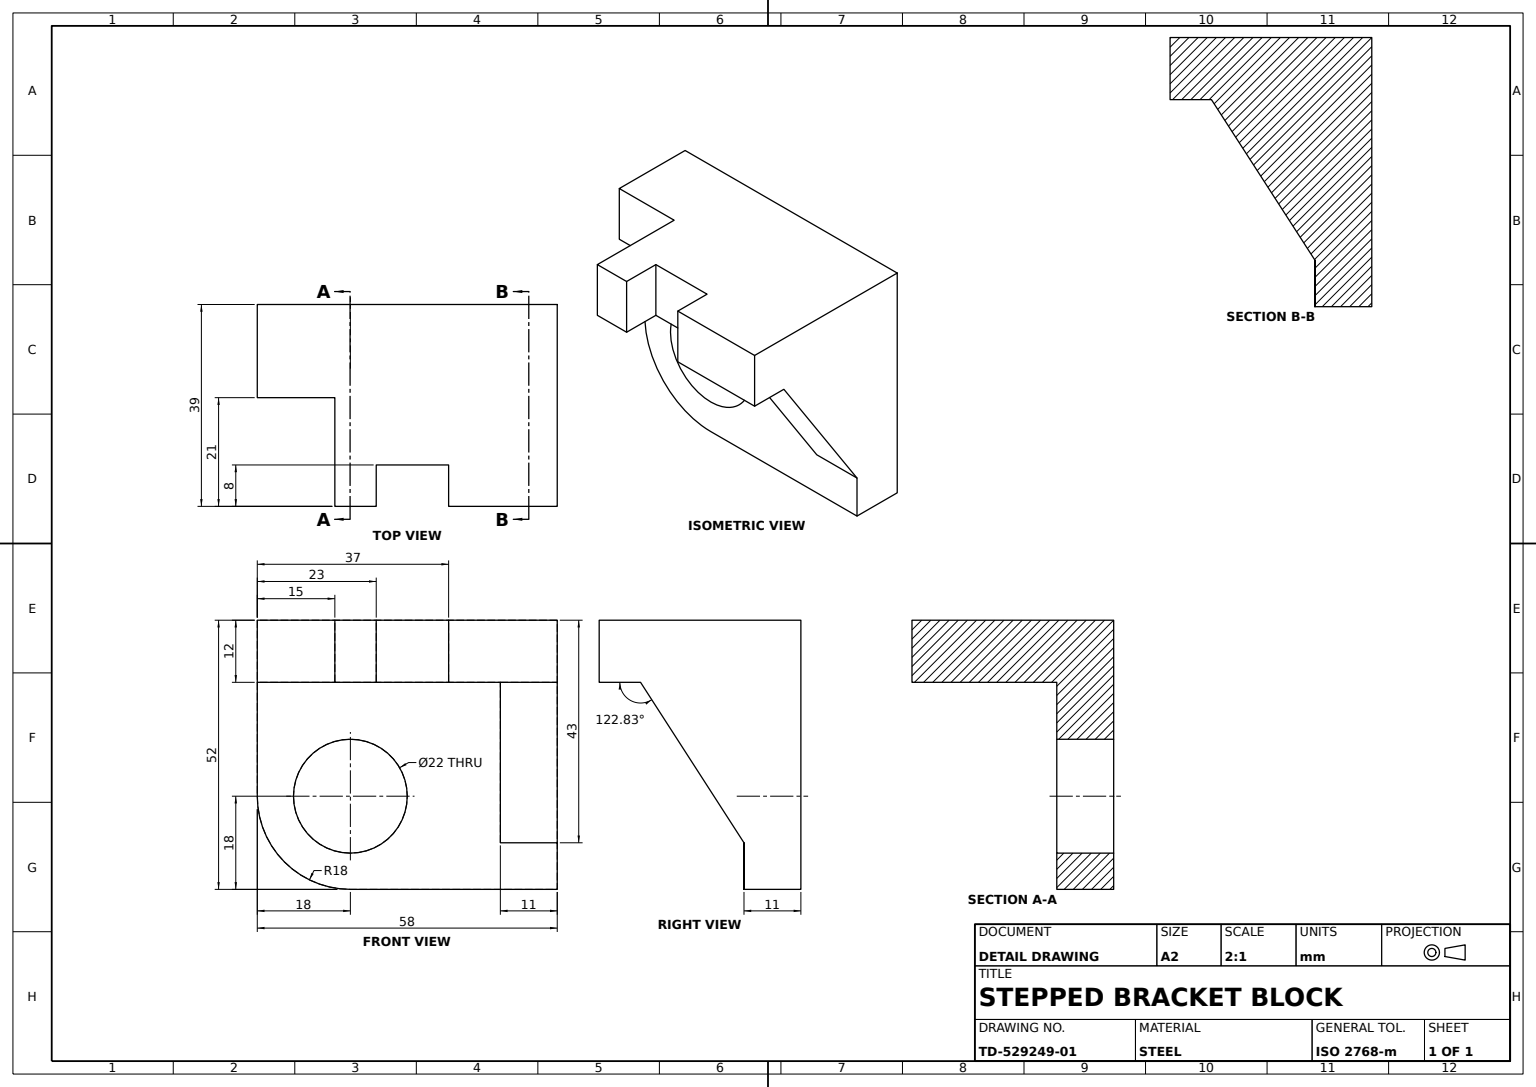
SolidWorks part; units mm, degrees
material "Plain Carbon Steel"
ref_plane "Front Plane" through (0, 0, 0) normal (0, 0, 1) x (1, 0, 0)
ref_plane "Top Plane" through (0, 0, 0) normal (0, 1, 0) x (1, 0, 0)
ref_plane "Right Plane" through (0, 0, 0) normal (1, 0, 0) x (0, 0, -1)
sketch "Base Block Profile" plane through (0, 0, 0) normal (0, 0, 1) x (1, 0, 0)
  line L1 (58, 0) -> (58, -52)
  line L2 (0, 0) -> (0, -34)
  line L3 (0, 0) -> (58, 0)
  line L5 (58, -52) -> (18, -52)
  arc A0 (0, -34) -> (18, -52) centre (18, -34) ccw
  dimension "D1" = 18
  dimension "D2" = 58
  dimension "D3" = 52
extrude "Base Block" add sketch "Base Block Profile" along normal blind 11
sketch "Top Plate Profile" plane through (0, 0, 0) normal (0, 1, 0) x (1, 0, 0)
  line L0 (58, -11) -> (58, -39)
  line L1 (58, -39) -> (37, -39)
  line L2 (37, -39) -> (37, -31)
  line L3 (37, -31) -> (23, -31)
  line L4 (0, -11) -> (0, -18)
  line L5 (0, -18) -> (15, -18)
  line L6 (15, -18) -> (15, -39)
  line L7 (15, -39) -> (23, -39)
  line L8 (23, -39) -> (23, -31)
  line L9 (58, -11) -> (0, -11)
  line L10 (0, -11) -> (0, 0) construction
  line L11 (58, 0) -> (0, 0) construction
  dimension "D1" = 15
  dimension "D2" = 23
  dimension "D3" = 37
  dimension "D4" = 18
extrude "Top Plate" add sketch "Top Plate Profile" against normal blind 12
sketch "Gusset Profile" plane through (58, 0, 0) normal (1, 0, 0) x (0, 0, -1)
  line L0 (-11, -12) -> (-31, -12)
  line L1 (-39, -12) -> (-11, -12) construction
  line L2 (-11, -12) -> (-11, -43)
  line L3 (-11, -52) -> (-11, -12) construction
  line L4 (-11, -43) -> (-31, -12)
  line L5 (0, -52) -> (0, 0) construction
  line L6 (-39, 0) -> (0, 0) construction
  dimension "D1" = 31
  dimension "D2" = 43
extrude "Gusset Rib" add sketch "Gusset Profile" against normal blind 11
sketch "Cut Ø22 Profile" plane through (0, 0, 11) normal (0, 0, 1) x (1, 0, 0)
  circle A0 centre (18, -34) radius 11
  dimension "D1" = 22
  dimension "D2" = 22
extrude "Cut Ø22" cut sketch "Cut Ø22 Profile" against normal blind 11
